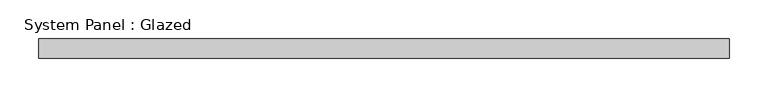
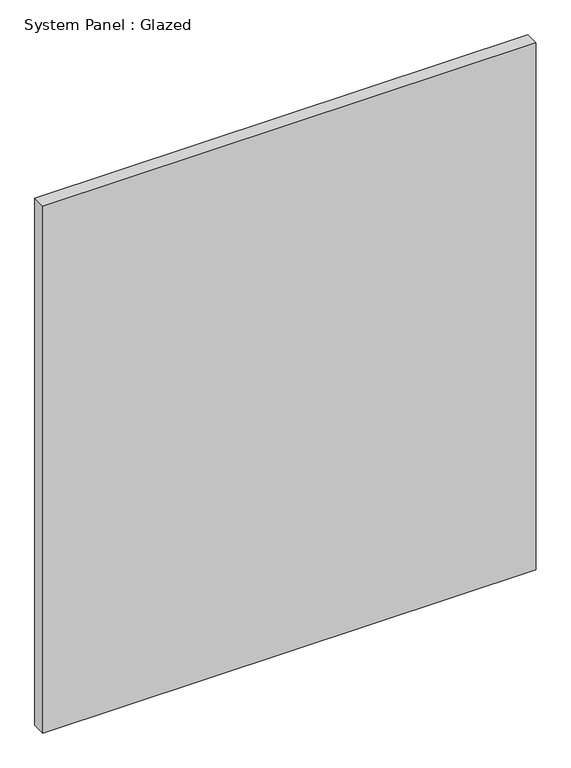
"""IFC4 building model written with IfcOpenShell, lengths in millimetres: plate geometry, System Panel : Glazed."""

from ifc_helpers import new_model, si_unit, origin, origin_with_axes, place, context, project, spatial, polyline, outline, extrude, source, transform, mapped, element, save


def system_panel_glazed_014df054(model_context):
    return source(origin(), model_context, "Body", "SweptSolid", [
        extrude(outline(polyline([(447.675, 19.05), (-447.675, 19.05), (-447.675, 44.45), (447.675, 44.45), (447.675, 19.05)])), origin_with_axes(), (0.0, 0.0, 1.0), 1010.9026335),
    ])


if __name__ == "__main__":
    model = new_model("IFC4")
    model_context = context("Model", 3, world=origin())
    ifc_project = project(units=[si_unit("LENGTHUNIT", "METRE", prefix="MILLI")], contexts=[model_context])
    site = spatial("IfcSite", under=ifc_project)
    building = spatial("IfcBuilding", under=site)
    placement = place(None, origin())
    system_panel_glazed_shape = system_panel_glazed_014df054(model_context)
    element("IfcPlate", 1, ObjectType="System Panel : Glazed", at=placement, inside=building, context=model_context, shape_type="MappedRepresentation", body=[
        mapped(system_panel_glazed_shape, transform((0.0, 0.0, 0.0), x_axis=(1.0, 0.0, 0.0), y_axis=(0.0, 1.0, 0.0), z_axis=(0.0, 0.0, 1.0))),
    ])
    save(model, "model.ifc")

# Revit data of these elements
# Type "System Panel : Glazed"
#   Construction Type Id = "GSP4R"
#   Analytic Construction = "1/8 in Pilkington single glazing"
#   Visual Light Transmittance = 0.9
#   Solar Heat Gain Coefficient = 0.86
#   Heat Transfer Coefficient (U) = 1.18115 BTU/(h·ft²·°F)
#   Define Thermal Properties by = 1
# Element 1 (IfcPlate, "System Panel : Glazed")
#   Materials on its faces: "Glass"
# Materials
#   "Glass": class "Glass", colour RGB 0 128 192, transparency 0.75, Description = "Soda Lime Glass", Cost = 0
